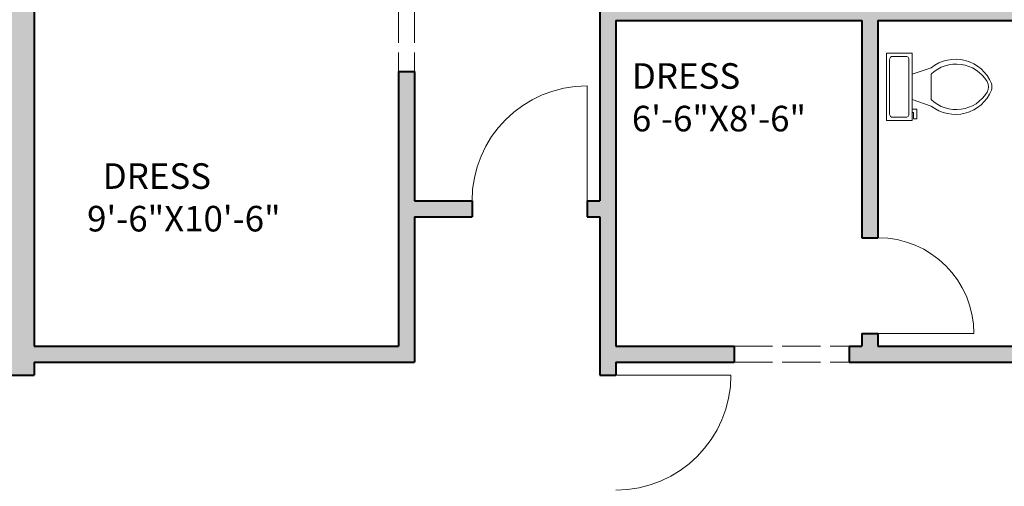
# Model space of a CAD drawing. Units: inches. Extents: x 2330 to 3943, y 1763 to 3461.
# Tile 26 of 40: x 2973 to 3281, y 2829 to 2975. Entities that reach past the tile are written whole.
import ezdxf

# ---------------------------------------------------------------- set-up
doc = ezdxf.new("R2010")
doc.units = ezdxf.units.IN
doc.linetypes.add('ACAD_ISO02W100', pattern=[15, 12, -3])
for name, color, linetype, lineweight in [('A-AREA-IDEN', 7, 'Continuous', 18), ('A-DOOR', 4, 'Continuous', 18), ('A-FLOR-FIXT', 8, 'Continuous', 18), ('A-WALL', 7, 'Continuous', 40), ('A-WALL-OVHD', 7, 'ACAD_ISO02W100', 18), ('A-WALL-PATT', 252, 'Continuous', 13)]:
    doc.layers.add(name, color=color, linetype=linetype, lineweight=lineweight)
doc.styles.get("Standard").update_dxf_attribs({"font": 'arial.ttf'})

# ---------------------------------------------------------------- blocks, each defined once
blk = doc.blocks.new('*U9')
for p, q in [((9.5, -6), (9.5, -2)), ((-10, -8.5), (-8, -8.5)), ((-10, -9.5), (-10, -8.5)), ((-8, -8.5), (-8, -8)), ((-7, -8), (-7, -9.5)), ((-4, -8), (-6, -14)), ((4, -8), (6, -14)), ((-7, -9.5), (-10, -9.5)), ((4, -14), (-4, -14))]:
    blk.add_line(p, q)
blk.add_lwpolyline([(10.5, -8), (10.5, 0), (-10.5, 0), (-10.5, -8)], close=True)
for points in [[(-9.5, -2), (-9.5, -6)], [(8.5, -1), (-8.5, -1)], [(-8.5, -7), (8.5, -7)]]:
    blk.add_lwpolyline(points)
for centre, radius, start, end in [((-8.62, -1.88), 0.884, 81.8699, 188.1301), ((8.62, -1.88), 0.884, 351.8699, 98.1301), ((-8.62, -6.12), 0.884, 171.8699, 278.1301), ((8.62, -6.12), 0.884, 261.8699, 8.1301), ((3.52, -21.58), 12.17, 141.4691, 247.9714), ((4.2, -21.82), 11.33, 136.3677, 238.9468), ((-3.52, -21.58), 12.17, 292.0284, 38.5307), ((-4.2, -21.82), 11.33, 301.053, 43.6321), ((0, -27.88), 4, 245.7318, 294.2682), ((0, -29), 4, 254.8605, 285.1395)]:
    blk.add_arc(centre, radius, start, end)
blk = doc.blocks.new('DOOR-SINGLE-36IN')
blk.add_line((0, 0), (-36, 0))
blk.add_arc((0, 0), 36, 180, 270)
blk = doc.blocks.new('DOOR-SINGLE-30IN')
blk.add_line((0, 0), (0, 30))
blk.add_arc((0, 0), 30, 90, 180)

msp = doc.modelspace()

# ---------------------------------------------------------------- hatches: boundary and pattern name
at = {"layer": 'A-WALL-PATT'}
h = msp.add_hatch(color=256, dxfattribs=at)
h.dxf.hatch_style = 1
h.paths.add_polyline_path([(3022.6605, 3162.6524), (2968.6605, 3162.6524), (2968.6605, 3083.6524), (2916.6605, 3083.6524), (2916.6605, 3074.6524), (2968.6605, 3074.6524), (2968.6605, 2863.6524), (2977.6605, 2863.6524), (2977.6605, 2867.6524), (3096.6605, 2867.6524), (3096.6605, 2913.1524), (3114.6605, 2913.1524), (3114.6605, 2918.1524), (3096.6605, 2918.1524), (3096.6605, 2958.6524), (3091.6605, 2958.6524), (3091.6605, 2872.6524), (2977.6605, 2872.6524), (2977.6605, 2998.6524), (3057.6605, 2998.6524), (3057.6605, 3003.6524), (2977.6605, 3003.6524), (2977.6605, 3153.6524), (3022.6605, 3153.6524)])
h = msp.add_hatch(color=256, dxfattribs=at)
h.dxf.hatch_style = 1
h.paths.add_polyline_path([(3241.6605, 2974.6524), (3376.7746, 2974.6524, -0.16828569), (3398.3014, 2935.4254), (3407.174, 2936.9344, 0.12044914), (3392.5913, 2970.6524), (3455.6605, 2970.6524), (3455.6605, 3018.6524), (3446.6605, 3018.6524), (3446.6605, 2979.6524), (3275.6605, 2979.6524), (3275.6605, 3018.6524), (3270.6605, 3018.6524), (3270.6605, 2979.6524), (3154.6605, 2979.6524), (3154.6605, 2918.1524), (3150.6605, 2918.1524), (3150.6605, 2913.1524), (3154.6605, 2913.1524), (3154.6605, 2863.6524), (3159.6605, 2863.6524), (3159.6605, 2867.6524), (3196.6605, 2867.6524), (3196.6605, 2872.6524), (3159.6605, 2872.6524), (3159.6605, 2974.6524), (3236.6605, 2974.6524), (3236.6605, 2906.6524), (3241.6605, 2906.6524)])
h = msp.add_hatch(color=256, dxfattribs=at)
h.dxf.hatch_style = 1
h.paths.add_polyline_path([(3387.1394, 2870.8379, 0.10459296), (3403.8352, 2898.1524), (3395.3511, 2901.1556, -0.12790871), (3376.0739, 2872.6524), (3241.6605, 2872.6524), (3241.6605, 2876.6524), (3236.6605, 2876.6524), (3236.6605, 2872.6524), (3232.6605, 2872.6524), (3232.6605, 2867.6524), (3378.6605, 2867.6524, -0.07524693), (3407.8539, 2780.6064), (3416.7189, 2782.159, 0.07442358)])

# ---------------------------------------------------------------- linework, layer by layer
at = {"layer": 'A-WALL'}
for p, q in [((2977.6605, 2998.6524), (2977.6605, 2872.6524)), ((3154.6605, 2979.6524), (3154.6605, 2918.1524)), ((3159.6605, 2974.6524), (3236.6605, 2974.6524)), ((3159.6605, 2974.6524), (3159.6605, 2872.6524)), ((3236.6605, 2974.6524), (3236.6605, 2906.6524)), ((3241.6605, 2974.6524), (3241.6605, 2906.6524)), ((3241.6605, 2974.6524), (3376.7746, 2974.6524)), ((3091.6605, 2958.6524), (3096.6605, 2958.6524)), ((3091.6605, 2958.6524), (3091.6605, 2872.6524)), ((3096.6605, 2958.6524), (3096.6605, 2918.1524)), ((3096.6605, 2918.1524), (3114.6605, 2918.1524)), ((3114.6605, 2918.1524), (3114.6605, 2913.1524)), ((3150.6605, 2918.1524), (3150.6605, 2913.1524)), ((3150.6605, 2918.1524), (3154.6605, 2918.1524)), ((3096.6605, 2913.1524), (3114.6605, 2913.1524)), ((3096.6605, 2913.1524), (3096.6605, 2867.6524)), ((3150.6605, 2913.1524), (3154.6605, 2913.1524)), ((3154.6605, 2913.1524), (3154.6605, 2863.6524)), ((3236.6605, 2906.6524), (3241.6605, 2906.6524)), ((3236.6605, 2876.6524), (3241.6605, 2876.6524)), ((3236.6605, 2876.6524), (3236.6605, 2872.6524)), ((3241.6605, 2876.6524), (3241.6605, 2872.6524)), ((2977.6605, 2872.6524), (3091.6605, 2872.6524)), ((3159.6605, 2872.6524), (3196.6605, 2872.6524)), ((3196.6605, 2872.6524), (3196.6605, 2867.6524)), ((3232.6605, 2872.6524), (3232.6605, 2867.6524)), ((3232.6605, 2872.6524), (3236.6605, 2872.6524)), ((3241.6605, 2872.6524), (3376.0739, 2872.6524)), ((2977.6605, 2867.6524), (3096.6605, 2867.6524)), ((2977.6605, 2867.6524), (2977.6605, 2863.6524)), ((3159.6605, 2867.6524), (3196.6605, 2867.6524)), ((3159.6605, 2867.6524), (3159.6605, 2863.6524)), ((3232.6605, 2867.6524), (3378.6605, 2867.6524)), ((2968.6605, 2863.6524), (2977.6605, 2863.6524)), ((3154.6605, 2863.6524), (3159.6605, 2863.6524))]:
    msp.add_line(p, q, dxfattribs=at)
at = {"layer": 'A-WALL-OVHD'}
for p, q in [((3091.6605, 2994.6524), (3091.6605, 2958.6524)), ((3096.6605, 2994.6524), (3096.6605, 2958.6524)), ((3196.6605, 2872.6524), (3232.6605, 2872.6524)), ((3196.6605, 2867.6524), (3232.6605, 2867.6524))]:
    msp.add_line(p, q, dxfattribs=at)

# ---------------------------------------------------------------- block references
at = {"layer": 'A-DOOR'}
for name, p, rotation in [('DOOR-SINGLE-36IN', (3150.6605, 2918.1524), 269.9999999999989), ('DOOR-SINGLE-30IN', (3241.6605, 2876.6524), 270.0000000000004)]:
    msp.add_blockref(name, p, dxfattribs=dict(at, rotation=rotation))
at = {"layer": 'A-DOOR', "extrusion": (0, 0, -1), "zscale": -1}
msp.add_blockref('DOOR-SINGLE-36IN', (-3159.6605, 2863.6524), dxfattribs=at)
at = {"layer": 'A-FLOR-FIXT', "rotation": 90}
msp.add_blockref('*U9', (3244.3074, 2953.8645), dxfattribs=at)

# ---------------------------------------------------------------- texts
at = {"layer": 'A-AREA-IDEN', "char_height": 8, "attachment_point": 1}
for s, width, insert in [('DRESS\\P6\'-6"X8\'-6"', 66.36581, (3164.6771, 2961.2666)), ('  DRESS\\P9\'-6"X10\'-6"', 89.990069, (2994.2514, 2929.9404))]:
    msp.add_mtext_dynamic_manual_height_columns(s, width=width, gutter_width=12.5, heights=[0], dxfattribs=dict(at, insert=insert))

doc.saveas('drawing.dxf')
